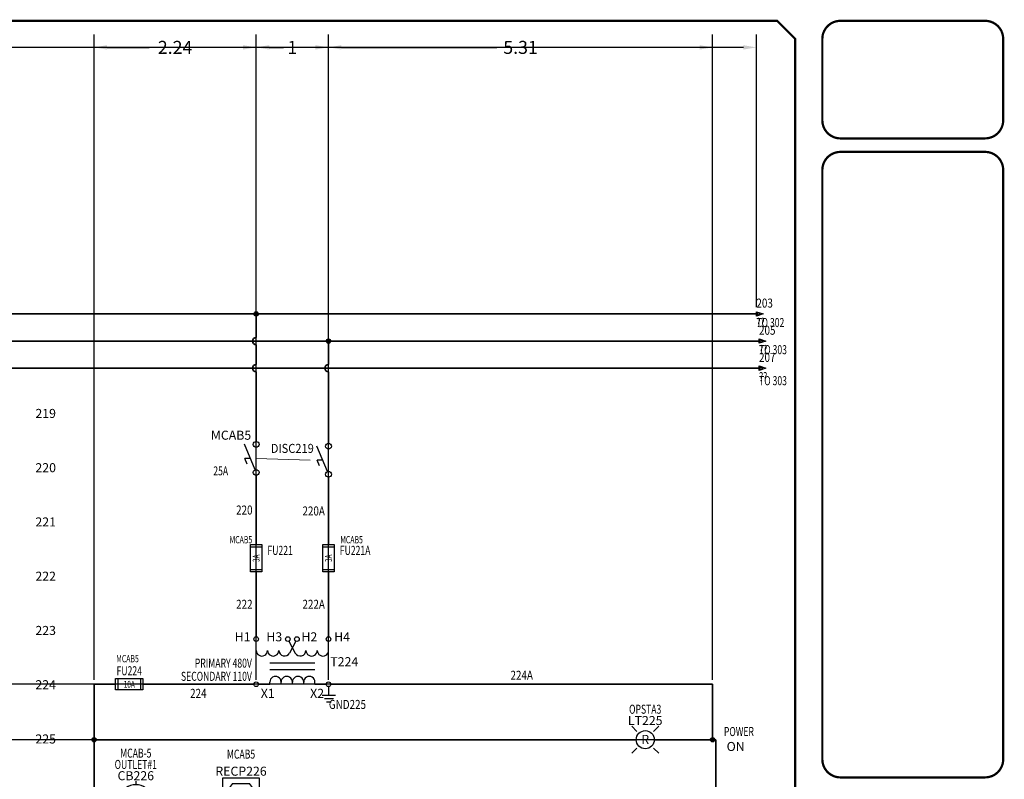
# Model space of a CAD drawing. Extents: x 0 to 33.5, y 0 to 22.4.
# Tile 8 of 8: x 19.9 to 33.5, y 11.9 to 22.4. Entities that reach past the tile are written whole.
import ezdxf
from ezdxf.enums import TextEntityAlignment as Align

# ---------------------------------------------------------------- set-up
doc = ezdxf.new("R2010")
doc.units = 0
doc.header["$MEASUREMENT"] = 0
for name, color, linetype, lineweight in [('A-ANNO-DIMS', 2, 'Continuous', 18), ('E-ANNO-TEXT', 3, 'Continuous', 18), ('LINK', 9, 'Continuous', 18), ('MISC', 7, 'Continuous', 13), ('SYMS', 7, 'Continuous', 25), ('TITLE', 7, 'Continuous', 35), ('WIRENO', 72, 'Continuous', 18), ('WIRES', 7, 'Continuous', 35)]:
    doc.layers.add(name, color=color, linetype=linetype, lineweight=lineweight)
for name, color, linetype in [('DESC', 150, 'Continuous'), ('LOC', 8, 'Continuous'), ('TAGS', 150, 'Continuous'), ('TERMS', 123, 'Continuous'), ('WIREREF', 52, 'Continuous'), ('XREF', 7, 'Continuous'), ('XREFCHILD', 134, 'Continuous')]:
    doc.layers.add(name, color=color, linetype=linetype)
doc.styles.add('ITALIC', font='ITALIC')
doc.styles.add('SIMPLEX', font='SIMPLEX')
doc.styles.add('WD', font='romans.shx')
doc.dimstyles.get("Standard").update_dxf_attribs({"dimtxt": 0.18, "dimasz": 0.18, "dimexe": 0.18, "dimexo": 0.0625, "dimgap": 0.09, "dimtad": 0, "dimtih": 1, "dimtoh": 1, "dimdec": 4, "dimzin": 0, "dimdsep": 46, "dimtxsty": 'Standard', "dimcen": 0.09, "dimadec": 0, "dimazin": 0, "dimtfac": 1, "dimtdec": 4, "dimtofl": 0, "dimtmove": 0, "dimatfit": 3, "dimfxl": 1, "dimtolj": 1, "dimtzin": 0, "dimarcsym": 0})

# ---------------------------------------------------------------- blocks, each defined once
blk = doc.blocks.new('NO_NUM_acade_title')
at = {"layer": 'TITLE'}
blk.add_line((30.594, 22.177), (30.594, 20.781), dxfattribs=at)
at = {"layer": 'TITLE', "const_width": 0.0312}
blk.add_lwpolyline([(30.594, 0.281), (30.594, 22.177), (30.344, 22.427), (0.281, 22.427), (0.031, 22.177), (0.031, 0.281), (0.281, 0.031), (30.344, 0.031)], close=True, dxfattribs=at)
for points in [[(31.219, 22.427, 0.414214), (30.969, 22.177, 0.414214)], [(33.469, 22.177, 0.414214), (33.219, 22.427, 0.414214)], [(30.969, 21.052, 0.414214), (31.219, 20.802, 0.414214)], [(33.219, 20.802, 0.414214), (33.469, 21.052, 0.414214)], [(31.219, 20.615, 0.414214), (30.969, 20.365, 0.414214)], [(33.469, 20.365, 0.414214), (33.219, 20.615, 0.414214)], [(30.969, 12.219, 0.414214), (31.219, 11.969, 0.414214)], [(33.219, 11.969, 0.414214), (33.469, 12.219, 0.414214)]]:
    blk.add_lwpolyline(points, format="xyb", dxfattribs=at)
for points in [[(33.219, 22.427), (31.219, 22.427)], [(30.969, 22.177), (30.969, 21.052)], [(33.469, 22.177), (33.469, 21.052)], [(33.219, 20.802), (31.219, 20.802)], [(33.219, 20.615), (31.219, 20.615)], [(30.969, 20.365), (30.969, 12.219)], [(33.469, 20.365), (33.469, 12.219)], [(31.219, 11.969), (33.219, 11.969)]]:
    blk.add_lwpolyline(points, dxfattribs=at)
at = {"layer": 'TITLE', "style": 'ITALIC'}
for tag, height, p in [('TITLE#1', 0.125, (32.156, 3.406)), ('TITLE#2', 0.125, (32.156, 3.204)), ('TITLE#3', 0.125, (32.156, 3.001)), ('TITLE#4', 0.125, (32.156, 2.799)), ('DWG#', 0.2, (32.156, 0.826))]:
    blk.add_attdef(tag, text='', height=height, dxfattribs=at).set_placement(p, align=Align.CENTER)
at = {"layer": 'TITLE', "style": 'SIMPLEX'}
blk.add_attdef('CAD#', (30.826, 1.958), '', height=0.0938, rotation=90, dxfattribs=at)
at = {"layer": 'TITLE'}
for tag, p, height, style in [('JOB#', (31.464, 1.644), 0.0938, 'SIMPLEX'), ('SCALE', (31.353, 1.344), 0.0938, 'SIMPLEX'), ('DATE', (32.408, 1.344), 0.0938, 'SIMPLEX'), ('SHTS', (32.532, 0.25), 0.2, 'ITALIC')]:
    blk.add_attdef(tag, p, '', height=height, dxfattribs=dict(at, style=style))
at = {"layer": 'TITLE', "style": 'ITALIC'}
blk.add_attdef('SH#', text='', height=0.2, dxfattribs=at).set_placement((31.881, 0.25), align=Align.RIGHT)
at = {"layer": 'TITLE', "flags": 9}
blk.add_attdef('WD_TB', (31.219, 0.031), '', height=0.125, dxfattribs=at)
blk = doc.blocks.new('WD_MLRH')
at = {"style": 'WD'}
blk.add_attdef('RUNGFIRST', text='', height=0.125, dxfattribs=at).set_placement((-0.25, 0), align=Align.MIDDLE_RIGHT)
at = {"style": 'WD', "flags": 1}
for tag, p in [('RUNGHORV', (-0.25, -0.127)), ('WIREMODE', (-0.25, -0.281)), ('RUNGDIST', (-0.25, -0.2)), ('RUNGCNT', (-0.25, -0.237)), ('RUNGINC', (-0.25, -0.163)), ('WIRE-START', (-0.25, -0.356)), ('WIRE-GSUF', (-0.25, -0.396)), ('WIREFMT', (-0.25, -0.321)), ('PH3SPACE', (-0.25, -0.437))]:
    blk.add_attdef(tag, text='', height=0.025, dxfattribs=at).set_placement(p, align=Align.RIGHT)
blk = doc.blocks.new('WDDOT')
for radius in [0.03, 0.0187, 0.00929]:
    blk.add_circle((0, 0), radius)
blk = doc.blocks.new('HXF1D')
for p, q in [((-0.5, -0.156), (-0.5, -0.032)), ((-0.048, -0.028), (0.04, -0.193)), ((0.047, -0.029), (-0.04, -0.193)), ((0.5, -0.156), (0.5, -0.032)), ((-0.312, -0.328), (0.312, -0.328)), ((-0.312, -0.422), (0.312, -0.422)), ((-0.469, -0.625), (-0.312, -0.625)), ((-0.312, -0.625), (-0.312, -0.594)), ((-0.156, -0.625), (-0.156, -0.594)), ((0, -0.625), (0, -0.594)), ((0.156, -0.625), (0.156, -0.594)), ((0.312, -0.625), (0.312, -0.594)), ((0.312, -0.625), (0.467, -0.625))]:
    blk.add_line(p, q)
for centre in [(-0.501, 0), (-0.063, 0), (0.062, 0), (0.499, 0), (-0.501, -0.625), (0.499, -0.625)]:
    blk.add_circle(centre, 0.0322)
for centre, start, end in [((-0.422, -0.156), 179.999, 0), ((-0.266, -0.156), 179.999, 0), ((-0.109, -0.156), 179.999, 331.9287), ((0.109, -0.156), 208.0713, 0.001), ((0.266, -0.156), 180, 0.001), ((0.422, -0.156), 180, 0.001), ((-0.234, -0.594), 0.001, 180.002), ((-0.078, -0.594), 0.001, 180.002), ((0.078, -0.594), 0.001, 180.002), ((0.234, -0.594), 0.001, 180.002)]:
    blk.add_arc(centre, 0.0781, start, end)
at = {"style": 'WD', "flags": 8}
for tag, p in [('TERM01', (-0.578, -0.031)), ('TERM02', (-0.141, -0.031))]:
    blk.add_attdef(tag, text='', height=0.125, dxfattribs=at).set_placement(p, align=Align.RIGHT)
at = {"style": 'WD'}
for tag, p, height, flags in [('X4TERM01', (-0.533, 0), 0.0125, 1), ('X2TERM01', (-0.501, 0.032), 0.0125, 1), ('X2TERM02', (-0.063, 0.032), 0.0125, 1), ('X2TERM03', (0.062, 0.032), 0.0125, 1), ('TERM03', (0.125, -0.031), 0.125, 8), ('X2TERM04', (0.499, 0.032), 0.0125, 1), ('X1TERM04', (0.531, 0), 0.0125, 1), ('TERM04', (0.578, -0.031), 0.125, 8), ('FAMILY', (0.46, -0.372), 0.01, 9), ('X4TERM05', (-0.533, -0.625), 0.0125, 1), ('X8TERM05', (-0.501, -0.657), 0.0125, 1), ('X8TERM06', (0, -0.632), 0.0125, 1), ('X8TERM07', (0.499, -0.657), 0.0125, 1), ('X1TERM07', (0.531, -0.625), 0.0125, 1)]:
    blk.add_attdef(tag, p, '', height=height, dxfattribs=dict(at, flags=flags))
at = {"style": 'WD', "width": 0.7}
for tag, p in [('INST', (-0.56, -0.181)), ('LOC', (-0.56, -0.351)), ('DESC1', (-0.56, -0.507)), ('DESC2', (-0.56, -0.664))]:
    blk.add_attdef(tag, text='', height=0.125, dxfattribs=at).set_placement(p, align=Align.RIGHT)
at = {"style": 'WD'}
blk.add_attdef('TAG1', (0.524, -0.375), '', height=0.125, dxfattribs=at)
at = {"style": 'WD', "flags": 9}
for tag, p in [('CAT', (0.485, -0.4)), ('ASSYCODE', (0.483, -0.438)), ('MFG', (0.484, -0.42))]:
    blk.add_attdef(tag, text='', height=0.01, dxfattribs=at).set_placement(p, align=Align.CENTER)
at = {"style": 'WD', "width": 0.7}
blk.add_attdef('RATING1', (0.556, -0.531), '', height=0.125, dxfattribs=at)
at = {"style": 'WD', "flags": 8}
for tag, p in [('TERM06', (-0.031, -0.688)), ('TERM07', (0.438, -0.688))]:
    blk.add_attdef(tag, text='', height=0.125, dxfattribs=at).set_placement(p, align=Align.TOP_RIGHT)
blk.add_attdef('TERM05', text='', height=0.125, dxfattribs=at).set_placement((-0.438, -0.688), align=Align.TOP_LEFT)
blk = doc.blocks.new('VDS11')
for p, q in [((-0.016, -0.157), (-0.163, 0.195)), ((-0.081, 0), (-0.156, 0)), ((-0.124, -0.078), (-0.156, 0))]:
    blk.add_line(p, q)
for centre in [(0, 0.194), (0, -0.194)]:
    blk.add_circle(centre, 0.0403)
at = {"style": 'WD'}
for tag, width, p in [('INST', 0.7, (-0.391, 0.312)), ('LOC', 0.7, (-0.391, 0.125)), ('TAG1', 0.9, (-0.388, -0.054)), ('RATING1', 0.7, (-0.388, -0.234)), ('DESC1', 0.7, (-0.387, -0.422)), ('DESC2', 0.7, (-0.388, -0.609))]:
    blk.add_attdef(tag, text='', height=0.125, dxfattribs=dict(at, width=width)).set_placement(p, align=Align.RIGHT)
for tag, height, flags, p in [('TERM01', 0.125, 8, (-0.069, 0.258)), ('CONTACT', 0.0125, 9, (-0.083, -0.067)), ('FAMILY', 0.0125, 9, (-0.1, -0.046)), ('MFG', 0.0125, 9, (-0.1, -0.11)), ('CAT', 0.0125, 9, (-0.1, -0.091))]:
    blk.add_attdef(tag, text='', height=height, dxfattribs=dict(at, flags=flags)).set_placement(p, align=Align.RIGHT)
at = {"style": 'WD', "flags": 1}
for tag, p in [('X2TERM01', (0, 0.234)), ('X8TERM02', (0, -0.234))]:
    blk.add_attdef(tag, p, '', height=0.0125, dxfattribs=at)
at = {"style": 'WD'}
for tag, p in [('X4LINK', (-0.254, 0)), ('X1LINK', (0, 0))]:
    blk.add_attdef(tag, p, '', height=0.0125, dxfattribs=at)
at = {"style": 'WD', "width": 0.7}
blk.add_attdef('XREF', (0.161, -0.047), '', height=0.125, dxfattribs=at)
at = {"style": 'WD', "flags": 9}
blk.add_attdef('ASSYCODE', text='', height=0.0125, dxfattribs=at).set_placement((-0.115, -0.137), align=Align.CENTER)
at = {"style": 'WD', "flags": 8}
blk.add_attdef('TERM02', text='', height=0.125, dxfattribs=at).set_placement((-0.051, -0.267), align=Align.TOP_RIGHT)
blk = doc.blocks.new('VFU1')
for p, q in [((-0.078, -0.188), (-0.078, 0.188)), ((-0.078, 0.188), (0.078, 0.188)), ((-0.078, 0.156), (0.078, 0.156)), ((0.078, 0.188), (0.078, -0.188)), ((-0.078, -0.156), (0.078, -0.156)), ((0.078, -0.188), (-0.078, -0.188))]:
    blk.add_line(p, q)
at = {"style": 'WD', "width": 0.7}
for tag, p in [('INST', (0.156, 0.359)), ('LOC', (0.156, 0.203)), ('TAG1', (0.156, 0.047)), ('DESC1', (0.156, -0.172)), ('DESC2', (0.156, -0.328)), ('DESC3', (0.156, -0.484))]:
    blk.add_attdef(tag, p, '', height=0.125, dxfattribs=at)
at = {"style": 'WD', "width": 0.7, "flags": 8}
blk.add_attdef('TERM01', text='', height=0.1, dxfattribs=at).set_placement((-0.055, 0.207), align=Align.RIGHT)
at = {"style": 'WD', "width": 0.7}
blk.add_attdef('RATING1', text='', height=0.0938, rotation=90, dxfattribs=at).set_placement((0, 0), align=Align.MIDDLE_CENTER)
at = {"style": 'WD', "flags": 1}
for tag, p in [('X2TERM01', (0, 0.188)), ('X8TERM02', (0, -0.188))]:
    blk.add_attdef(tag, p, '', height=0.0109, dxfattribs=at)
at = {"style": 'WD'}
for tag, p in [('X4LINK', (-0.125, 0)), ('X1LINK', (0.141, 0))]:
    blk.add_attdef(tag, p, '', height=0.01, dxfattribs=at)
at = {"style": 'WD', "flags": 9}
blk.add_attdef('ASSYCODE', text='', height=0.01, dxfattribs=at).set_placement((-0.098, -0.108), align=Align.CENTER)
for tag, p in [('FAMILY', (-0.08, -0.036)), ('MFG', (-0.08, -0.088)), ('CAT', (-0.08, -0.073))]:
    blk.add_attdef(tag, text='', height=0.01, dxfattribs=at).set_placement(p, align=Align.RIGHT)
at = {"style": 'WD', "width": 0.7, "flags": 8}
blk.add_attdef('TERM02', text='', height=0.1, dxfattribs=at).set_placement((-0.041, -0.213), align=Align.TOP_RIGHT)
blk = doc.blocks.new('HFU1')
for p, q in [((-0.188, -0.078), (-0.188, 0.078)), ((-0.188, 0.078), (0.188, 0.078)), ((-0.156, 0.078), (-0.156, -0.078)), ((0.156, 0.078), (0.156, -0.078)), ((0.188, 0.078), (0.188, -0.078)), ((0.188, -0.078), (-0.188, -0.078))]:
    blk.add_line(p, q)
at = {"style": 'WD', "width": 0.7}
for tag, p in [('INST', (0, 0.422)), ('LOC', (0, 0.266)), ('TAG1', (0, 0.125))]:
    blk.add_attdef(tag, text='', height=0.125, dxfattribs=at).set_placement(p, align=Align.CENTER)
at = {"style": 'WD', "flags": 9}
for tag, p in [('ASSYCODE', (0.157, 0.251)), ('MFG', (0.156, 0.083)), ('CAT', (0.156, 0.102))]:
    blk.add_attdef(tag, text='', height=0.01, dxfattribs=at).set_placement(p, align=Align.CENTER)
at = {"style": 'WD'}
for tag, p, height, flags in [('X4TERM01', (-0.188, 0), 0.0109, 1), ('FAMILY', (0.129, 0.108), 0.01, 9), ('X1TERM02', (0.188, 0), 0.0109, 1)]:
    blk.add_attdef(tag, p, '', height=height, dxfattribs=dict(at, flags=flags))
at = {"style": 'WD', "width": 0.7}
blk.add_attdef('RATING1', text='', height=0.0938, dxfattribs=at).set_placement((0, 0), align=Align.MIDDLE_CENTER)
at = {"style": 'WD'}
for tag, p in [('X2LINK', (0, 0.109)), ('X8LINK', (0, -0.109))]:
    blk.add_attdef(tag, p, '', height=0.01, dxfattribs=at)
at = {"style": 'WD', "width": 0.7, "flags": 8}
blk.add_attdef('TERM01', text='', height=0.1, dxfattribs=at).set_placement((-0.25, -0.016), align=Align.TOP_RIGHT)
blk.add_attdef('TERM02', text='', height=0.1, dxfattribs=at).set_placement((0.25, -0.016), align=Align.TOP_LEFT)
at = {"style": 'WD', "width": 0.7}
for tag, p in [('DESC1', (0.047, -0.234)), ('DESC2', (0.047, -0.391)), ('DESC3', (0.047, -0.547))]:
    blk.add_attdef(tag, text='', height=0.125, dxfattribs=at).set_placement(p, align=Align.MIDDLE_LEFT)
blk = doc.blocks.new('HGND2')
for p, q in [((0.125, 0), (0, 0)), ((0.125, 0.09375), (0.125, -0.09375)), ((0.171875, 0.0625), (0.171875, -0.0625)), ((0.21875, 0.03125), (0.21875, -0.03125))]:
    blk.add_line(p, q)
at = {"style": 'WD', "width": 0.8}
for tag, p in [('INST', (0.25, 0.3125)), ('LOC', (0.25, 0.15625)), ('TAG1', (0.25, 0)), ('DESC1', (0.25, -0.15625)), ('DESC2', (0.25, -0.3125))]:
    blk.add_attdef(tag, text='', height=0.125, dxfattribs=at).set_placement(p, align=Align.MIDDLE_LEFT)
at = {"style": 'WD', "flags": 1}
for tag in ['ASSYCODE', 'X4TERM01', 'CAT', 'MFG', 'FAMILY']:
    blk.add_attdef(tag, (0, 0), '', height=0.01, dxfattribs=at)
blk = doc.blocks.new('HCB1')
blk.add_line((0, 0.173), (0, 0.126))
for centre in [(-0.155, 0), (0.155, 0)]:
    blk.add_circle(centre, 0.0322)
blk.add_arc((0, -0.109), 0.234, 53.1301, 126.8699)
at = {"style": 'WD', "width": 0.7}
for tag, p in [('INST', (0, 0.826)), ('LOC', (0, 0.656)), ('DESC1', (0, 0.5)), ('DESC2', (0, 0.344)), ('RATING1', (0, -0.188)), ('XREF', (0, -0.344))]:
    blk.add_attdef(tag, text='', height=0.125, dxfattribs=at).set_placement(p, align=Align.CENTER)
at = {"style": 'WD'}
blk.add_attdef('TAG1', text='', height=0.125, dxfattribs=at).set_placement((0, 0.188), align=Align.CENTER)
for tag, p in [('X2LINK', (0, 0.219)), ('X8LINK', (0, 0))]:
    blk.add_attdef(tag, p, '', height=0.01, dxfattribs=at)
for tag, p, height, flags in [('CONTACT', (0.205, 0.133), 0.01, 9), ('FAMILY', (0.205, 0.152), 0.01, 9), ('X4TERM01', (-0.188, 0), 0.0125, 1), ('X1TERM02', (0.188, 0), 0.0125, 1)]:
    blk.add_attdef(tag, p, '', height=height, dxfattribs=dict(at, flags=flags))
at = {"style": 'WD', "flags": 9}
for tag, p in [('ASSYCODE', (0.219, 0.062)), ('MFG', (0.228, 0.089)), ('CAT', (0.23, 0.108))]:
    blk.add_attdef(tag, text='', height=0.01, dxfattribs=at).set_placement(p, align=Align.CENTER)
at = {"style": 'WD', "flags": 8}
blk.add_attdef('TERM01', text='', height=0.125, dxfattribs=at).set_placement((-0.25, -0.031), align=Align.TOP_RIGHT)
blk.add_attdef('TERM02', text='', height=0.125, dxfattribs=at).set_placement((0.25, -0.031), align=Align.TOP_LEFT)
blk = doc.blocks.new('HCN1RDUP')
for p, q in [((-0.25, 0.219), (0.25, 0.219)), ((-0.25, -0.656), (-0.25, 0.219)), ((0.117, 0.14), (-0.117, 0.14)), ((0.25, 0.219), (0.25, -0.656)), ((-0.071, 0.071), (-0.071, -0.046)), ((0.07, 0.071), (0.07, -0.046)), ((-0.024, -0.093), (0.023, -0.093)), ((-0.024, -0.125), (-0.024, -0.093)), ((0.023, -0.093), (0.023, -0.125)), ((0.117, -0.187), (-0.117, -0.187)), ((0.117, -0.235), (-0.117, -0.235)), ((0.008, -0.14), (-0.009, -0.14)), ((-0.071, -0.304), (-0.071, -0.421)), ((0.07, -0.304), (0.07, -0.421)), ((-0.024, -0.468), (0.023, -0.468)), ((-0.024, -0.5), (-0.024, -0.468)), ((0.008, -0.515), (-0.009, -0.515)), ((0.023, -0.468), (0.023, -0.5)), ((0.25, -0.656), (-0.25, -0.656)), ((0.117, -0.562), (-0.117, -0.562))]:
    blk.add_line(p, q)
for centre, radius, start, end in [((0.039, -0.023), 0.226, 133.6028, 226.3972), ((-0.039, -0.023), 0.226, 313.6028, 46.3972), ((-0.009, -0.125), 0.015, 180, 270), ((0.008, -0.125), 0.015, 270, 0), ((0.039, -0.398), 0.226, 133.6028, 226.3972), ((-0.039, -0.398), 0.226, 313.6028, 46.3972), ((-0.009, -0.5), 0.015, 180, 270), ((0.008, -0.5), 0.015, 270, 0)]:
    blk.add_arc(centre, radius, start, end)
at = {"style": 'WD', "width": 0.7}
for tag, p in [('INST', (0, 0.875)), ('LOC', (0, 0.719)), ('DESC1', (0, 0.562)), ('DESC2', (0, 0.406))]:
    blk.add_attdef(tag, text='', height=0.125, dxfattribs=at).set_placement(p, align=Align.CENTER)
at = {"style": 'WD'}
blk.add_attdef('TAG1', text='', height=0.125, dxfattribs=at).set_placement((0, 0.25), align=Align.CENTER)
for tag, p, height, flags in [('FAMILY', (0.205, 0.152), 0.01, 9), ('X4TERM01', (-0.188, 0), 0.0125, 1), ('X1TERM02', (0.188, 0), 0.0125, 1), ('X8TERM03', (0, -0.14), 0.0125, 1), ('X4TERM04', (-0.188, -0.375), 0.0125, 1), ('X1TERM05', (0.188, -0.375), 0.0125, 1), ('X8TERM06', (0, -0.515), 0.0125, 1)]:
    blk.add_attdef(tag, p, '', height=height, dxfattribs=dict(at, flags=flags))
at = {"style": 'WD', "flags": 9}
for tag, p in [('ASSYCODE', (0.23, 0.071)), ('MFG', (0.228, 0.089)), ('CAT', (0.23, 0.108))]:
    blk.add_attdef(tag, text='', height=0.01, dxfattribs=at).set_placement(p, align=Align.CENTER)
at = {"style": 'WD', "flags": 8}
for tag, p in [('TERM01', (-0.281, -0.016)), ('TERM04', (-0.281, -0.391))]:
    blk.add_attdef(tag, text='', height=0.125, dxfattribs=at).set_placement(p, align=Align.TOP_RIGHT)
for tag, p in [('TERM02', (0.281, -0.016)), ('TERM05', (0.281, -0.391)), ('TERM06', (0.078, -0.688))]:
    blk.add_attdef(tag, text='', height=0.125, dxfattribs=at).set_placement(p, align=Align.TOP_LEFT)
at = {"style": 'WD', "width": 0.9}
blk.add_attdef('RATING1', text='', height=0.125, dxfattribs=at).set_placement((-0.281, -0.812), align=Align.RIGHT)
blk = doc.blocks.new('HSS2R')
for p, q in [((-0.115, 0.115), (-0.186, 0.186)), ((0.115, 0.115), (0.186, 0.186)), ((-0.115, -0.115), (-0.186, -0.186)), ((0.115, -0.115), (0.186, -0.186))]:
    blk.add_line(p, q)
blk.add_circle((0, 0), 0.125)
at = {"style": 'WD', "width": 0.7}
for tag, p in [('INST', (0, 0.528)), ('LOC', (0, 0.359)), ('XREF', (0, -0.312))]:
    blk.add_attdef(tag, text='', height=0.125, dxfattribs=at).set_placement(p, align=Align.CENTER)
at = {"style": 'WD'}
for tag, p in [('TAG2', (0, 0.202)), ('COLOR', (0, -0.058))]:
    blk.add_attdef(tag, text='', height=0.125, dxfattribs=at).set_placement(p, align=Align.CENTER)
at = {"style": 'WD', "flags": 9}
blk.add_attdef('FAMILY', text='', height=0.01, dxfattribs=at).set_placement((-0.005, 0.161), align=Align.CENTER)
at = {"style": 'WD'}
for tag, p in [('X2LINK', (0, 0.219)), ('X8LINK', (0, -0.219))]:
    blk.add_attdef(tag, p, '', height=0.01, dxfattribs=at)
at = {"style": 'WD', "flags": 1}
for tag, p in [('X4TERM01', (-0.125, 0)), ('X1TERM02', (0.125, 0))]:
    blk.add_attdef(tag, p, '', height=0.0125, dxfattribs=at)
at = {"style": 'WD', "flags": 8}
blk.add_attdef('TERM01', text='', height=0.125, dxfattribs=at).set_placement((-0.175, -0.031), align=Align.TOP_RIGHT)
blk.add_attdef('TERM02', text='', height=0.125, dxfattribs=at).set_placement((0.175, -0.031), align=Align.TOP_LEFT)
blk = doc.blocks.new('HA1S1')
for points in [[(0, 0), (0, 0.031), (0.094, 0), (0, -0.031), (0, 0)], [(0.011, 0.016), (0.011, -0.016), (0.058, 0), (0.011, 0.016)]]:
    blk.add_lwpolyline(points)
at = {"style": 'WD', "width": 0.8, "flags": 8}
blk.add_attdef('WIRENO', (0, 0.087), '', height=0.125, dxfattribs=at)
at = {"style": 'WD', "flags": 1}
for tag, p in [('SIGCODE', (-0.02, 0.047)), ('X4TERM01', (0, 0))]:
    blk.add_attdef(tag, p, '', height=0.01, dxfattribs=at)
at = {"style": 'WD', "width": 0.7}
for tag, p in [('XREF', (0, -0.181)), ('DESC1', (0, -0.356))]:
    blk.add_attdef(tag, p, '', height=0.125, dxfattribs=at)
blk = doc.blocks.new('WD_WNV')
at = {"style": 'WD', "width": 0.8}
blk.add_attdef('WIRENO', text='', height=0.125, dxfattribs=at).set_placement((-0.05, 0), align=Align.MIDDLE_RIGHT)
at = {"style": 'WD', "flags": 1}
for tag, p in [('W01USER', (-0.062, 0.094)), ('W02USER', (-0.062, 0.086)), ('W03USER', (-0.062, 0.078)), ('W04USER', (-0.062, 0.07)), ('W05USER', (-0.062, 0.062)), ('W06USER', (-0.062, 0.055)), ('W07USER', (-0.062, 0.047)), ('W08USER', (-0.062, 0.039)), ('W09USER', (-0.062, 0.031)), ('W10USER', (-0.062, 0.023))]:
    blk.add_attdef(tag, text='', height=0.005, dxfattribs=at).set_placement(p, align=Align.CENTER)
blk = doc.blocks.new('WD_WNH')
at = {"style": 'WD', "width": 0.8}
blk.add_attdef('WIRENO', text='', height=0.125, dxfattribs=at).set_placement((0, 0.062), align=Align.CENTER)
at = {"style": 'WD', "flags": 1}
for tag, p in [('W01USER', (0, 0.078)), ('W02USER', (0, 0.07)), ('W03USER', (0, 0.062)), ('W04USER', (0, 0.055)), ('W05USER', (0, 0.047)), ('W06USER', (0, 0.039)), ('W07USER', (0, 0.031)), ('W08USER', (0, 0.023)), ('W09USER', (0, 0.016)), ('W10USER', (0, 0.008))]:
    blk.add_attdef(tag, text='', height=0.005, dxfattribs=at).set_placement(p, align=Align.CENTER)
blk = doc.blocks.new('*D37')
at = {"layer": 'A-ANNO-DIMS', "color": 0, "lineweight": -2, "transparency": 16777216}
for p, q in [((3.125, 18.4375), (3.125, 22.239937)), ((30.05762, 18.46875), (30.05762, 22.239937)), ((3.305, 22.059937), (16.14131, 22.059937)), ((29.87762, 22.059937), (17.04131, 22.059937))]:
    blk.add_line(p, q, dxfattribs=at)
at = {"layer": 'A-ANNO-DIMS', "color": 0, "transparency": 16777216}
for points in [[(3.305, 22.089937), (3.305, 22.029937), (3.125, 22.059937)], [(29.87762, 22.089937), (29.87762, 22.029937), (30.05762, 22.059937)]]:
    blk.add_solid(points, dxfattribs=at)
at = {"layer": 'Defpoints', "color": 0, "transparency": 16777216}
for p in [(30.05762, 22.059937), (3.125, 18.375), (30.05762, 18.40625)]:
    blk.add_point(p, dxfattribs=at)
at = {"layer": 'A-ANNO-DIMS', "color": 0, "transparency": 16777216, "insert": (16.59131, 22.059937), "char_height": 0.18, "attachment_point": 5}
blk.add_mtext('\\A1;26.93', dxfattribs=at)
blk = doc.blocks.new('*D49')
at = {"layer": 'A-ANNO-DIMS', "color": 0, "lineweight": -2, "transparency": 16777216}
for p, q in [((20.901, 13.318), (20.901, 22.24)), ((23.142, 13.318), (23.142, 22.24)), ((21.081, 22.06), (21.662, 22.06)), ((22.962, 22.06), (22.382, 22.06))]:
    blk.add_line(p, q, dxfattribs=at)
at = {"layer": 'A-ANNO-DIMS', "color": 0, "transparency": 16777216}
for points in [[(21.081, 22.09), (21.081, 22.03), (20.901, 22.06)], [(22.962, 22.09), (22.962, 22.03), (23.142, 22.06)]]:
    blk.add_solid(points, dxfattribs=at)
at = {"layer": 'Defpoints', "color": 0, "transparency": 16777216}
for p in [(23.142, 22.06), (20.901, 13.256), (23.142, 13.256)]:
    blk.add_point(p, dxfattribs=at)
at = {"layer": 'A-ANNO-DIMS', "color": 0, "transparency": 16777216, "insert": (22.022, 22.06), "char_height": 0.18, "attachment_point": 5}
blk.add_mtext('\\A1;2.24', dxfattribs=at)
blk = doc.blocks.new('*D50')
at = {"layer": 'A-ANNO-DIMS', "color": 0, "lineweight": -2, "transparency": 16777216}
for p, q in [((23.142405, 13.318275), (23.142405, 22.239937)), ((24.142405, 13.318275), (24.142405, 22.239937)), ((23.322405, 22.059937), (23.522405, 22.059937)), ((23.962405, 22.059937), (23.762405, 22.059937))]:
    blk.add_line(p, q, dxfattribs=at)
at = {"layer": 'A-ANNO-DIMS', "color": 0, "transparency": 16777216}
for points in [[(23.322405, 22.089937), (23.322405, 22.029937), (23.142405, 22.059937)], [(23.962405, 22.089937), (23.962405, 22.029937), (24.142405, 22.059937)]]:
    blk.add_solid(points, dxfattribs=at)
at = {"layer": 'Defpoints', "color": 0, "transparency": 16777216}
for p in [(24.142405, 22.059937), (23.142405, 13.255775), (24.142405, 13.255775)]:
    blk.add_point(p, dxfattribs=at)
at = {"layer": 'A-ANNO-DIMS', "color": 0, "transparency": 16777216, "insert": (23.642405, 22.059937), "char_height": 0.18, "attachment_point": 5}
blk.add_mtext('\\A1;1', dxfattribs=at)
blk = doc.blocks.new('*D51')
at = {"layer": 'A-ANNO-DIMS', "color": 0, "lineweight": -2, "transparency": 16777216}
for p, q in [((24.142, 13.318), (24.142, 22.24)), ((29.452, 13.318), (29.452, 22.24)), ((24.322, 22.06), (26.467, 22.06)), ((29.272, 22.06), (27.127, 22.06))]:
    blk.add_line(p, q, dxfattribs=at)
at = {"layer": 'A-ANNO-DIMS', "color": 0, "transparency": 16777216}
for points in [[(24.322, 22.09), (24.322, 22.03), (24.142, 22.06)], [(29.272, 22.09), (29.272, 22.03), (29.452, 22.06)]]:
    blk.add_solid(points, dxfattribs=at)
at = {"layer": 'Defpoints', "color": 0, "transparency": 16777216}
for p in [(29.452, 22.06), (24.142, 13.256), (29.452, 13.256)]:
    blk.add_point(p, dxfattribs=at)
at = {"layer": 'A-ANNO-DIMS', "color": 0, "transparency": 16777216, "insert": (26.797, 22.06), "char_height": 0.18, "attachment_point": 5}
blk.add_mtext('\\A1;5.31', dxfattribs=at)
blk = doc.blocks.new('*D56')
at = {"layer": 'A-ANNO-DIMS', "color": 0, "lineweight": -2, "transparency": 16777216}
for p, q in [((29.389766, 13.255775), (1.48, 13.255775)), ((1.66, 13.075775), (1.66, 12.669774)), ((29.4322, 12.489774), (1.48, 12.489774)), ((1.66, 12.489774), (1.66, 12.309774)), ((1.66, 12.309774), (1.48, 12.309774))]:
    blk.add_line(p, q, dxfattribs=at)
at = {"layer": 'A-ANNO-DIMS', "color": 0, "transparency": 16777216}
for points in [[(1.63, 13.075775), (1.69, 13.075775), (1.66, 13.255775)], [(1.63, 12.669774), (1.69, 12.669774), (1.66, 12.489774)]]:
    blk.add_solid(points, dxfattribs=at)
at = {"layer": 'Defpoints', "color": 0, "transparency": 16777216}
for p in [(29.452266, 13.255775), (1.66, 12.489774), (29.4947, 12.489774)]:
    blk.add_point(p, dxfattribs=at)
at = {"layer": 'A-ANNO-DIMS', "color": 0, "transparency": 16777216, "insert": (1.045, 12.309774), "char_height": 0.18, "attachment_point": 5}
blk.add_mtext('\\A1;0.766', dxfattribs=at)
blk = doc.blocks.new('*D57')
at = {"layer": 'A-ANNO-DIMS', "color": 0, "lineweight": -2, "transparency": 16777216}
for p, q in [((29.4322, 12.489774), (1.48, 12.489774)), ((1.66, 12.309774), (1.66, 11.913516)), ((29.435818, 11.733516), (1.48, 11.733516)), ((1.66, 11.733516), (1.66, 11.553516)), ((1.66, 11.553516), (1.48, 11.553516))]:
    blk.add_line(p, q, dxfattribs=at)
at = {"layer": 'A-ANNO-DIMS', "color": 0, "transparency": 16777216}
for points in [[(1.63, 12.309774), (1.69, 12.309774), (1.66, 12.489774)], [(1.63, 11.913516), (1.69, 11.913516), (1.66, 11.733516)]]:
    blk.add_solid(points, dxfattribs=at)
at = {"layer": 'Defpoints', "color": 0, "transparency": 16777216}
for p in [(29.4947, 12.489774), (1.66, 11.733516), (29.498318, 11.733516)]:
    blk.add_point(p, dxfattribs=at)
at = {"layer": 'A-ANNO-DIMS', "color": 0, "transparency": 16777216, "insert": (1.135, 11.553516), "char_height": 0.18, "attachment_point": 5}
blk.add_mtext('\\A1;0.76', dxfattribs=at)
blk = doc.blocks.new('*D61')
at = {"layer": 'A-ANNO-DIMS', "color": 0, "lineweight": -2, "transparency": 16777216}
for p, q in [((23.088, 18.379), (1.48, 18.379)), ((1.66, 18.199), (1.66, 15.997)), ((1.66, 13.436), (1.66, 15.637)), ((20.838, 13.256), (1.48, 13.256))]:
    blk.add_line(p, q, dxfattribs=at)
at = {"layer": 'A-ANNO-DIMS', "color": 0, "transparency": 16777216}
for points in [[(1.63, 18.199), (1.69, 18.199), (1.66, 18.379)], [(1.63, 13.436), (1.69, 13.436), (1.66, 13.256)]]:
    blk.add_solid(points, dxfattribs=at)
at = {"layer": 'Defpoints', "color": 0, "transparency": 16777216}
for p in [(23.151, 18.379), (1.66, 13.256), (20.901, 13.256)]:
    blk.add_point(p, dxfattribs=at)
at = {"layer": 'A-ANNO-DIMS', "color": 0, "transparency": 16777216, "insert": (1.66, 15.817), "char_height": 0.18, "attachment_point": 5}
blk.add_mtext('\\A1;5.123', dxfattribs=at)

msp = doc.modelspace()

# ---------------------------------------------------------------- linework, layer by layer
at = {"layer": 'LINK'}
msp.add_lwpolyline([(23.1424, 16.3782), (23.8885, 16.3529)], dxfattribs=at)
at = {"layer": 'WIRES'}
for p, q in [((5.1875, 18.375), (30.0576, 18.375)), ((23.1424, 18.05), (23.1424, 18.375)), ((5.1875, 18), (30.0939, 18)), ((24.1424, 17.675), (24.1424, 18)), ((23.1424, 17.675), (23.1424, 17.95)), ((5.1875, 17.625), (30.0939, 17.625)), ((23.1424, 16.6126), (23.1424, 17.575)), ((24.1424, 16.5873), (24.1424, 17.575)), ((23.1424, 15.1855), (23.1424, 16.1438)), ((24.1424, 15.1855), (24.1424, 16.1186)), ((23.1424, 13.913), (23.1424, 14.8105)), ((24.1424, 13.913), (24.1424, 14.8105)), ((20.9008, 13.2558), (20.9008, 8.7023)), ((20.9008, 13.2558), (21.2004, 13.2558)), ((21.5754, 13.2558), (23.1102, 13.2558)), ((24.1746, 13.2558), (29.4523, 13.2558)), ((29.4523, 12.4898), (29.4523, 13.2558)), ((20.9008, 12.4898), (28.3955, 12.4898)), ((28.6455, 12.4898), (29.4947, 12.4898)), ((29.4947, 12.4898), (29.4947, 8.7023))]:
    msp.add_line(p, q, dxfattribs=at)
for centre in [(23.1424, 18), (23.1424, 17.625), (24.1424, 17.625)]:
    msp.add_arc(centre, 0.05, 90, 270, dxfattribs=at)

# ---------------------------------------------------------------- block references
at = {"layer": 'MISC'}
msp.add_blockref('WD_MLRH', (20.6248, 17), dxfattribs=at).add_auto_attribs({'RUNGFIRST': '219'})
at = {"layer": 'SYMS'}
ref = msp.add_blockref('HA1S1', (30.0576, 18.375), dxfattribs=at)
ref.add_attrib('DESC1', 'TO 302', (30.0576, 18.1938), dxfattribs={"layer": 'DESC', "height": 0.125, "style": 'WD', "width": 0.7})
ref.add_attrib('WIRENO', '203', (30.0576, 18.4625), dxfattribs={"layer": 'WIREREF', "height": 0.125, "style": 'WD', "width": 0.8, "flags": 8})
ref.add_attrib('XREF', '??', (30.0576, 18.1938), dxfattribs={"layer": 'XREF', "height": 0.125, "style": 'WD', "width": 0.7})
for name, p in [('WDDOT', (23.1424, 18.375)), ('WDDOT', (24.1424, 18)), ('VDS11', (24.1424, 16.3529)), ('WDDOT', (20.9008, 12.4898)), ('WDDOT', (29.4523, 12.4898))]:
    msp.add_blockref(name, p, dxfattribs=at)
ref = msp.add_blockref('HA1S1', (30.0939, 18), dxfattribs=at)
ref.add_attrib('DESC1', 'TO 303', (30.0939, 17.8188), dxfattribs={"layer": 'DESC', "height": 0.125, "style": 'WD', "width": 0.7})
ref.add_attrib('WIRENO', '205', (30.0939, 18.0875), dxfattribs={"layer": 'WIREREF', "height": 0.125, "style": 'WD', "width": 0.8, "flags": 8})
ref.add_attrib('XREF', '??', (30.0939, 17.8188), dxfattribs={"layer": 'XREF', "height": 0.125, "style": 'WD', "width": 0.7})
ref = msp.add_blockref('HA1S1', (30.0939, 17.625), dxfattribs=at)
ref.add_attrib('DESC1', 'TO 303', (30.0939, 17.3902), dxfattribs={"layer": 'DESC', "height": 0.125, "style": 'WD', "width": 0.7})
ref.add_attrib('WIRENO', '207', (30.0939, 17.7125), dxfattribs={"layer": 'WIREREF', "height": 0.125, "style": 'WD', "width": 0.8, "flags": 8})
ref.add_attrib('XREF', '??', (30.0939, 17.4438), dxfattribs={"layer": 'XREF', "height": 0.125, "style": 'WD', "width": 0.7})
ref = msp.add_blockref('VDS11', (23.1424, 16.3782), dxfattribs=at)
ref.add_attrib('TAG1', 'DISC219', dxfattribs={"layer": 'TAGS', "height": 0.125, "style": 'WD', "width": 0.9}).set_placement((23.9395, 16.4541), align=Align.RIGHT)
ref.add_attrib('TERM01', 'MCAB5', dxfattribs={"layer": 'TERMS', "height": 0.125, "style": 'WD', "flags": 8}).set_placement((23.0737, 16.6365), align=Align.RIGHT)
ref.add_attrib('RATING1', '25A', dxfattribs={"layer": 'MISC', "height": 0.125, "style": 'WD', "width": 0.7}).set_placement((22.7547, 16.1438), align=Align.RIGHT)
ref = msp.add_blockref('VFU1', (23.1424, 14.998), dxfattribs=at)
ref.add_attrib('TAG1', 'FU221', (23.2987, 15.0449), dxfattribs={"layer": 'TAGS', "height": 0.125, "style": 'WD', "width": 0.7})
ref.add_attrib('TERM01', 'MCAB5', dxfattribs={"layer": 'TERMS', "linetype": 'Continuous', "height": 0.1, "style": 'WD', "width": 0.7, "flags": 8}).set_placement((23.0874, 15.2047), align=Align.RIGHT)
ref.add_attrib('RATING1', '3A', dxfattribs={"layer": 'MISC', "height": 0.09375, "rotation": 90, "style": 'WD', "width": 0.7}).set_placement((23.1424, 14.998), align=Align.MIDDLE_CENTER)
ref = msp.add_blockref('VFU1', (24.1424, 14.998), dxfattribs=at)
ref.add_attrib('TAG1', 'FU221A', (24.2987, 15.0449), dxfattribs={"layer": 'TAGS', "height": 0.125, "style": 'WD', "width": 0.7})
ref.add_attrib('TERM01', 'MCAB5', dxfattribs={"layer": 'TERMS', "linetype": 'Continuous', "height": 0.1, "style": 'WD', "width": 0.7, "flags": 8}).set_placement((24.6175, 15.2047), align=Align.RIGHT)
ref.add_attrib('RATING1', '3A', dxfattribs={"layer": 'MISC', "height": 0.09375, "rotation": 90, "style": 'WD', "width": 0.7}).set_placement((24.1424, 14.998), align=Align.MIDDLE_CENTER)
ref = msp.add_blockref('HXF1D', (23.6434, 13.8808), dxfattribs=at)
ref.add_attrib('TERM02', 'H3', dxfattribs={"layer": 'TERMS', "linetype": 'Continuous', "height": 0.125, "style": 'WD', "flags": 8}).set_placement((23.5027, 13.8495), align=Align.RIGHT)
ref.add_attrib('TERM01', 'H1', dxfattribs={"layer": 'TERMS', "linetype": 'Continuous', "height": 0.125, "style": 'WD', "flags": 8}).set_placement((23.0652, 13.8495), align=Align.RIGHT)
ref.add_attrib('TERM04', 'H4', (24.2215, 13.8495), dxfattribs={"layer": 'TERMS', "linetype": 'Continuous', "height": 0.125, "style": 'WD', "flags": 8})
ref.add_attrib('TERM05', 'X1', dxfattribs={"layer": 'TERMS', "linetype": 'Continuous', "height": 0.125, "style": 'WD', "flags": 8}).set_placement((23.2059, 13.1933), align=Align.TOP_LEFT)
ref.add_attrib('TERM07', 'X2', dxfattribs={"layer": 'TERMS', "linetype": 'Continuous', "height": 0.125, "style": 'WD', "flags": 8}).set_placement((24.0809, 13.1933), align=Align.TOP_RIGHT)
ref.add_attrib('TAG1', 'T224', (24.1677, 13.5058), dxfattribs={"layer": 'TAGS', "height": 0.125, "style": 'WD'})
ref.add_attrib('DESC1', 'PRIMARY 480V', dxfattribs={"layer": 'DESC', "height": 0.125, "style": 'WD', "width": 0.7}).set_placement((23.0835, 13.486), align=Align.RIGHT)
ref.add_attrib('DESC2', 'SECONDARY 110V', dxfattribs={"layer": 'DESC', "height": 0.125, "style": 'WD', "width": 0.7}).set_placement((23.0835, 13.3036), align=Align.RIGHT)
ref.add_attrib('TERM03', 'H2', (23.7684, 13.8495), dxfattribs={"layer": 'TERMS', "linetype": 'Continuous', "height": 0.125, "style": 'WD', "flags": 8})
ref = msp.add_blockref('HFU1', (21.3879, 13.2558), dxfattribs=at)
ref.add_attrib('RATING1', '10A', dxfattribs={"layer": 'MISC', "height": 0.09375, "style": 'WD', "width": 0.7}).set_placement((21.3879, 13.2558), align=Align.MIDDLE_CENTER)
ref.add_attrib('TERM01', 'MCAB5', dxfattribs={"layer": 'TERMS', "linetype": 'Continuous', "height": 0.1, "style": 'WD', "width": 0.7, "flags": 8}).set_placement((21.5202, 13.6602), align=Align.TOP_RIGHT)
ref.add_attrib('TAG1', 'FU224', dxfattribs={"layer": 'TAGS', "height": 0.125, "style": 'WD', "width": 0.7}).set_placement((21.3879, 13.3808), align=Align.CENTER)
ref = msp.add_blockref('HGND2', (24.1474, 13.2274), dxfattribs=dict(at, rotation=270))
ref.add_attrib('TAG1', 'GND225', dxfattribs={"layer": 'TAGS', "height": 0.125, "style": 'WD', "width": 0.8}).set_placement((24.1474, 12.9774), align=Align.MIDDLE_LEFT)
ref = msp.add_blockref('HSS2R', (28.5205, 12.4901), dxfattribs=at)
ref.add_attrib('XREF', 'POWER', dxfattribs={"layer": 'XREFCHILD', "height": 0.125, "style": 'WD', "width": 0.7}).set_placement((29.8157, 12.5402), align=Align.CENTER)
ref.add_attrib('LOC', 'OPSTA3', dxfattribs={"layer": 'LOC', "height": 0.125, "style": 'WD', "width": 0.7}).set_placement((28.5205, 12.8487), align=Align.CENTER)
ref.add_attrib('TERM01', 'ON', dxfattribs={"layer": 'TERMS', "linetype": 'Continuous', "height": 0.125, "style": 'WD', "flags": 8}).set_placement((29.8956, 12.4587), align=Align.TOP_RIGHT)
ref.add_attrib('TAG2', 'LT225', dxfattribs={"layer": 'TAGS', "height": 0.125, "style": 'WD'}).set_placement((28.5205, 12.6925), align=Align.CENTER)
ref.add_attrib('COLOR', 'R', dxfattribs={"layer": 'MISC', "height": 0.125, "style": 'WD'}).set_placement((28.5205, 12.4318), align=Align.CENTER)
ref = msp.add_blockref('HCB1', (21.4786, 11.7421), dxfattribs=at)
ref.add_attrib('RATING1', '15A', dxfattribs={"layer": 'MISC', "height": 0.125, "style": 'WD', "width": 0.7}).set_placement((21.4786, 11.6685), align=Align.CENTER)
ref.add_attrib('DESC2', 'OUTLET#1', dxfattribs={"layer": 'DESC', "height": 0.125, "style": 'WD', "width": 0.7}).set_placement((21.4786, 12.0858), align=Align.CENTER)
ref.add_attrib('DESC1', 'MCAB-5', dxfattribs={"layer": 'DESC', "height": 0.125, "style": 'WD', "width": 0.7}).set_placement((21.4786, 12.2421), align=Align.CENTER)
ref.add_attrib('TAG1', 'CB226', dxfattribs={"layer": 'TAGS', "height": 0.125, "style": 'WD'}).set_placement((21.4786, 11.9296), align=Align.CENTER)
ref = msp.add_blockref('HCN1RDUP', (22.9333, 11.7421), dxfattribs=at)
ref.add_attrib('LOC', 'MCAB5', dxfattribs={"layer": 'LOC', "height": 0.125, "style": 'WD', "width": 0.7}).set_placement((22.9333, 12.2282), align=Align.CENTER)
ref.add_attrib('TAG1', 'RECP226', dxfattribs={"layer": 'TAGS', "height": 0.125, "style": 'WD'}).set_placement((22.9333, 11.9921), align=Align.CENTER)
at = {"layer": 'TITLE'}
msp.add_blockref('NO_NUM_acade_title', (0, 0), dxfattribs=at)
at = {"layer": 'WIRENO'}
ref = msp.add_blockref('WD_WNV', (23.1424, 15.6647), dxfattribs=at)
ref.add_attrib('WIRENO', '220', dxfattribs={"linetype": 'Continuous', "height": 0.125, "style": 'WD', "width": 0.8}).set_placement((23.0924, 15.6647), align=Align.MIDDLE_RIGHT)
ref = msp.add_blockref('WD_WNV', (24.1424, 15.6521), dxfattribs=at)
ref.add_attrib('WIRENO', '220A', dxfattribs={"linetype": 'Continuous', "height": 0.125, "style": 'WD', "width": 0.8}).set_placement((24.0924, 15.6521), align=Align.MIDDLE_RIGHT)
ref = msp.add_blockref('WD_WNV', (23.1424, 14.3618), dxfattribs=at)
ref.add_attrib('WIRENO', '222', dxfattribs={"linetype": 'Continuous', "height": 0.125, "style": 'WD', "width": 0.8}).set_placement((23.0924, 14.3618), align=Align.MIDDLE_RIGHT)
ref = msp.add_blockref('WD_WNV', (24.1424, 14.3618), dxfattribs=at)
ref.add_attrib('WIRENO', '222A', dxfattribs={"linetype": 'Continuous', "height": 0.125, "style": 'WD', "width": 0.8}).set_placement((24.0924, 14.3618), align=Align.MIDDLE_RIGHT)
ref = msp.add_blockref('WD_WNH', (26.8134, 13.2558), dxfattribs=at)
ref.add_attrib('WIRENO', '224A', dxfattribs={"linetype": 'Continuous', "height": 0.125, "style": 'WD', "width": 0.8}).set_placement((26.8134, 13.3183), align=Align.CENTER)
ref = msp.add_blockref('WD_WNH', (22.3428, 13.2558), dxfattribs=at)
ref.add_attrib('WIRENO', '224', dxfattribs={"linetype": 'Continuous', "height": 0.125, "style": 'WD', "width": 0.8}).set_placement((22.3428, 13.1933), align=Align.TOP_CENTER)

# ---------------------------------------------------------------- texts
at = {"layer": 'E-ANNO-TEXT', "style": 'WD'}
for s, p in [('220', (20.3748, 16.25)), ('221', (20.3748, 15.5)), ('222', (20.3748, 14.75)), ('223', (20.3748, 14)), ('224', (20.3748, 13.25)), ('225', (20.3748, 12.5))]:
    msp.add_text(s, height=0.125, dxfattribs=at).set_placement(p, align=Align.MIDDLE_RIGHT)

# ---------------------------------------------------------------- dimensions: what is measured, and where the dimension line sits
at = {"layer": 'A-ANNO-DIMS'}
for base, p1, p2, override, picture, middle in [((30.0576, 22.0599), (3.125, 18.375), (30.0576, 18.4062), {"dimdec": 2, "dimlfac": 1, "dimrnd": 0, "dimzin": 0, "dimdsep": 46, "dimlunit": 2}, '*D37', (16.5913, 22.0599)), ((23.1424, 22.0599), (20.9008, 13.2558), (23.1424, 13.2558), {"dimdec": 2, "dimlfac": 1, "dimrnd": 0, "dimzin": 0, "dimdsep": 46, "dimlunit": 2}, '*D49', (22.0216, 22.0599)), ((24.1424, 22.0599), (23.1424, 13.2558), (24.1424, 13.2558), {"dimdec": 0, "dimlfac": 1, "dimrnd": 0, "dimzin": 0, "dimdsep": 46, "dimlunit": 2}, '*D50', (23.6424, 22.0599)), ((29.4523, 22.0599), (24.1424, 13.2558), (29.4523, 13.2558), {"dimdec": 2, "dimlfac": 1, "dimrnd": 0, "dimzin": 0, "dimdsep": 46, "dimlunit": 2}, '*D51', (26.7973, 22.0599))]:
    dim = msp.add_linear_dim(base=base, p1=p1, p2=p2, dimstyle='Standard', override=override, dxfattribs=at)
    dim.commit()
    dim.dimension.update_dxf_attribs({"geometry": picture, "text_midpoint": middle})
for base, p1, p2, override, picture, middle in [((1.66, 13.2558), (23.151, 18.3786), (20.9008, 13.2558), {"dimdec": 3, "dimlfac": 1, "dimrnd": 0, "dimzin": 0, "dimdsep": 46, "dimlunit": 2}, '*D61', (1.66, 15.8172)), ((1.66, 12.4898), (29.4523, 13.2558), (29.4947, 12.4898), {"dimdec": 3, "dimlfac": 1, "dimrnd": 0, "dimzin": 0, "dimdsep": 46, "dimlunit": 2}, '*D56', (1.045, 12.3098)), ((1.66, 11.7335), (29.4947, 12.4898), (29.4983, 11.7335), {"dimdec": 2, "dimlfac": 1, "dimrnd": 0, "dimzin": 0, "dimdsep": 46, "dimlunit": 2}, '*D57', (1.135, 11.5535))]:
    dim = msp.add_linear_dim(base=base, p1=p1, p2=p2, angle=90, dimstyle='Standard', override=override, dxfattribs=at)
    dim.commit()
    dim.dimension.update_dxf_attribs({"geometry": picture, "text_midpoint": middle})

doc.saveas('drawing.dxf')
